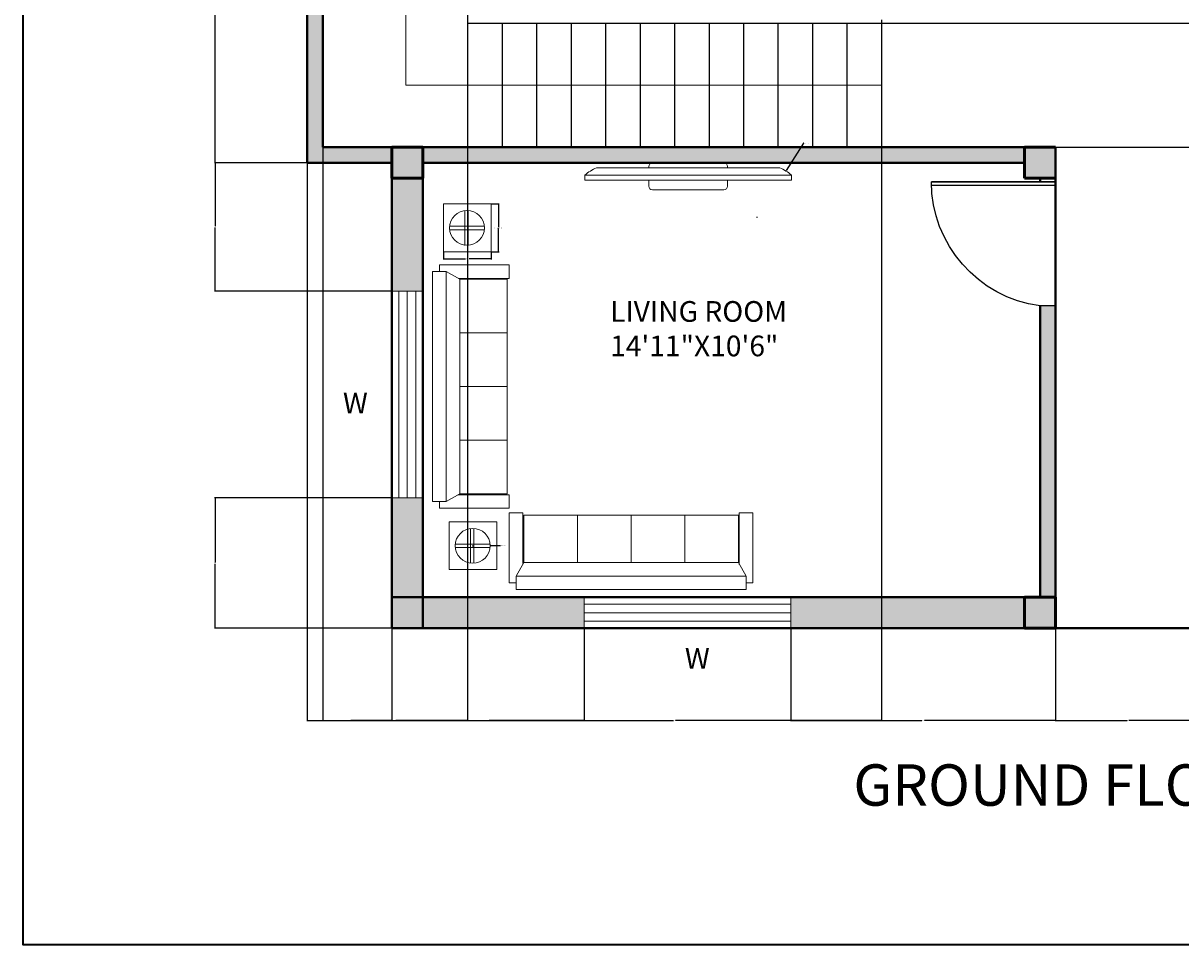
# Model space of a CAD drawing. Units: inches. Extents: x 25176543 to 25177243, y 80295576 to 80296086.
# Tile 1 of 11: x 25176543 to 25176879, y 80295576 to 80295843. Entities that reach past the tile are written whole.
import ezdxf

# ---------------------------------------------------------------- set-up
doc = ezdxf.new("R2010")
doc.units = ezdxf.units.IN
doc.header["$MEASUREMENT"] = 0
for name, color, linetype, lineweight in [('A-ANNO-DIMS', 2, 'Continuous', 18), ('A-ANNO-IDEN', 7, 'Continuous', 18), ('A-ANNO-SYMB', 7, 'Continuous', 18), ('A-ANNO-TTLB', 7, 'Continuous', 35), ('A-AREA-IDEN', 7, 'Continuous', 18), ('A-COLS', 7, 'Continuous', 50), ('A-COLS-PATT', 251, 'Continuous', 13), ('A-DOOR', 3, 'Continuous', 25), ('A-EQPM', 8, 'Continuous', 18), ('A-FLOR-STRS', 7, 'Continuous', 25), ('A-GLAZ', 4, 'Continuous', 18), ('A-WALL', 7, 'Continuous', 40), ('A-WALL-PATT', 146, 'Continuous', 13), ('furniture', 31, 'Continuous', 13)]:
    doc.layers.add(name, color=color, linetype=linetype, lineweight=lineweight)
doc.styles.get("Standard").update_dxf_attribs({"font": 'arial.ttf'})
doc.dimstyles.get("Standard").update_dxf_attribs({"dimtxt": 0.18, "dimasz": 0.18, "dimexe": 0.18, "dimexo": 0.0625, "dimgap": 0.09, "dimtad": 0, "dimtih": 1, "dimtoh": 1, "dimdec": 4, "dimzin": 0, "dimdsep": 46, "dimtxsty": 'Standard', "dimcen": 0.09, "dimadec": 0, "dimazin": 0, "dimtfac": 1, "dimtdec": 4, "dimtofl": 0, "dimtmove": 0, "dimatfit": 3, "dimfxl": 1, "dimtolj": 1, "dimtzin": 0, "dimarcsym": 0})

# ---------------------------------------------------------------- blocks, each defined once
blk = doc.blocks.new('SOFA-FOUR-SEAT')
for p, q in [((1.96, 70.61), (22.23, 70.61)), ((1.96, 70.61), (1.96, 68.65)), ((22.23, 66.69), (22.23, 70.61)), ((0, 68.65), (0, 1.96)), ((3.92, 68.65), (0, 68.65)), ((3.92, 68.65), (3.92, 1.96)), ((3.92, 68.65), (7.85, 66.44)), ((7.54, 66.69), (22.23, 66.69)), ((21.58, 50.87), (7.85, 50.87)), ((21.58, 35.31), (7.85, 35.31)), ((21.58, 19.74), (7.85, 19.74)), ((7.85, 4.17), (3.92, 1.96)), ((7.29, 3.92), (22.23, 3.92)), ((22.23, 3.92), (22.23, 0)), ((3.92, 1.96), (0, 1.96)), ((1.96, 1.96), (1.96, 0)), ((1.96, 0), (22.23, 0))]:
    blk.add_line(p, q)
blk.add_lwpolyline([(7.85, 66.44), (7.85, 4.17), (21.58, 4.17), (21.58, 66.44)], close=True)
blk = doc.blocks.new('END-TABLE')
for p, q in [((13.85, 13.86), (0, 13.86)), ((0, 13.86), (0, 0)), ((13.85, 0), (13.85, 13.86)), ((6.16, 11.93), (6.16, 1.84)), ((7.16, 11.93), (7.16, 1.84)), ((1.79, 7.4), (11.88, 7.4)), ((1.79, 6.4), (11.88, 6.4)), ((0, 0), (13.85, 0))]:
    blk.add_line(p, q)
blk.add_circle((6.83, 6.93), 5.05)
blk = doc.blocks.new('WIN-60IN')
for p, q in [((0, 9), (0, 0)), ((60, 9), (0, 9)), ((0, 9), (0, 4.5)), ((60, 7), (0, 7)), ((60, 0), (60, 9)), ((0, 4.5), (60, 4.5)), ((0, 2), (60, 2)), ((0, 0), (60, 0))]:
    blk.add_line(p, q)
blk = doc.blocks.new('DOOR-36IN')
for p, q in [((36, 37), (31.5, 37)), ((36, 1), (36, 37)), ((0, 2), (36, 2)), ((36, 1), (0, 1)), ((0, 1), (36, 1)), ((36, 0), (36, 1))]:
    blk.add_line(p, q)
blk.add_arc((36.32, 1), 36.32, 97.6281, 180)
blk = doc.blocks.new('COLUMN-9IN-SQ')
for p, q in [((9, 9), (0, 9)), ((0, 9), (0, 0)), ((9, 0), (9, 9)), ((0, 0), (9, 0))]:
    blk.add_line(p, q)
blk = doc.blocks.new('*D36')
at = {"layer": 'A-ANNO-DIMS', "color": 0, "lineweight": -2, "transparency": 16777216}
for p, q in [((25176678.7, 80295790.86), (25176680.9, 80295790.86)), ((25176680.72, 80295790.68), (25176680.72, 80295784.11)), ((25176680.72, 80295777.17), (25176680.72, 80295783.74)), ((25176678.7, 80295776.99), (25176680.9, 80295776.99))]:
    blk.add_line(p, q, dxfattribs=at)
at = {"layer": 'A-ANNO-DIMS', "color": 0, "transparency": 16777216}
for points in [[(25176680.69, 80295790.68), (25176680.75, 80295790.68), (25176680.72, 80295790.86)], [(25176680.69, 80295777.17), (25176680.75, 80295777.17), (25176680.72, 80295776.99)]]:
    blk.add_solid(points, dxfattribs=at)
at = {"layer": 'Defpoints', "color": 0, "transparency": 16777216}
for p in [(25176678.64, 80295790.86), (25176680.72, 80295790.86), (25176678.64, 80295776.99)]:
    blk.add_point(p, dxfattribs=at)
at = {"layer": 'A-ANNO-DIMS', "color": 0, "transparency": 16777216, "insert": (25176680.72, 80295783.92), "char_height": 0.18, "attachment_point": 5}
blk.add_mtext('\\A1;END TABLE 14 TYP.', dxfattribs=at)
blk = doc.blocks.new('*D37')
at = {"layer": 'A-ANNO-DIMS', "color": 0, "lineweight": -2, "transparency": 16777216}
for p, q in [((25176664.79, 80295776.93), (25176664.79, 80295774.74)), ((25176664.97, 80295774.92), (25176671.19, 80295774.92)), ((25176678.46, 80295774.92), (25176672.23, 80295774.92)), ((25176678.64, 80295776.93), (25176678.64, 80295774.74))]:
    blk.add_line(p, q, dxfattribs=at)
at = {"layer": 'A-ANNO-DIMS', "color": 0, "transparency": 16777216}
for points in [[(25176664.97, 80295774.95), (25176664.97, 80295774.89), (25176664.79, 80295774.92)], [(25176678.46, 80295774.95), (25176678.46, 80295774.89), (25176678.64, 80295774.92)]]:
    blk.add_solid(points, dxfattribs=at)
at = {"layer": 'Defpoints', "color": 0, "transparency": 16777216}
for p in [(25176664.79, 80295776.99), (25176678.64, 80295776.99), (25176678.64, 80295774.92)]:
    blk.add_point(p, dxfattribs=at)
at = {"layer": 'A-ANNO-DIMS', "color": 0, "transparency": 16777216, "insert": (25176671.71, 80295774.92), "char_height": 0.18, "attachment_point": 5}
blk.add_mtext('\\A1;14 TYP.', dxfattribs=at)
blk = doc.blocks.new('*D50')
at = {"layer": 'A-ANNO-DIMS', "color": 0, "lineweight": -2, "transparency": 16777216}
for p, q in [((25176625.3, 80295802.74), (25176625.3, 80295640.87)), ((25176649.8, 80295802.74), (25176649.8, 80295640.87)), ((25176625.48, 80295641.05), (25176637.23, 80295641.05)), ((25176649.62, 80295641.05), (25176637.88, 80295641.05))]:
    blk.add_line(p, q, dxfattribs=at)
at = {"layer": 'A-ANNO-DIMS', "color": 0, "transparency": 16777216}
for points in [[(25176625.48, 80295641.08), (25176625.48, 80295641.02), (25176625.3, 80295641.05)], [(25176649.62, 80295641.08), (25176649.62, 80295641.02), (25176649.8, 80295641.05)]]:
    blk.add_solid(points, dxfattribs=at)
at = {"layer": 'Defpoints', "color": 0, "transparency": 16777216}
for p in [(25176625.3, 80295802.8), (25176649.8, 80295802.8), (25176649.8, 80295641.05)]:
    blk.add_point(p, dxfattribs=at)
at = {"layer": 'A-ANNO-DIMS', "color": 0, "transparency": 16777216, "insert": (25176637.55, 80295641.05), "char_height": 0.18, "attachment_point": 5}
blk.add_mtext('\\A1;24.5', dxfattribs=at)
blk = doc.blocks.new('*D51')
at = {"layer": 'A-ANNO-DIMS', "color": 0, "lineweight": -2, "transparency": 16777216}
for p, q in [((25176625.24, 80295890.3), (25176598.37, 80295890.3)), ((25176598.55, 80295890.12), (25176598.55, 80295846.73)), ((25176598.55, 80295802.98), (25176598.55, 80295846.37)), ((25176625.24, 80295802.8), (25176598.37, 80295802.8))]:
    blk.add_line(p, q, dxfattribs=at)
at = {"layer": 'A-ANNO-DIMS', "color": 0, "transparency": 16777216}
for points in [[(25176598.52, 80295890.12), (25176598.58, 80295890.12), (25176598.55, 80295890.3)], [(25176598.52, 80295802.98), (25176598.58, 80295802.98), (25176598.55, 80295802.8)]]:
    blk.add_solid(points, dxfattribs=at)
at = {"layer": 'Defpoints', "color": 0, "transparency": 16777216}
for p in [(25176598.55, 80295890.3), (25176625.3, 80295890.3), (25176625.3, 80295802.8)]:
    blk.add_point(p, dxfattribs=at)
at = {"layer": 'A-ANNO-DIMS', "color": 0, "transparency": 16777216, "insert": (25176598.55, 80295846.55), "char_height": 0.18, "attachment_point": 5}
blk.add_mtext('\\A1;87.5', dxfattribs=at)
blk = doc.blocks.new('*D52')
at = {"layer": 'A-ANNO-DIMS', "color": 0, "lineweight": -2, "transparency": 16777216}
for p, q in [((25176842.3, 80295667.74), (25176842.3, 80295640.87)), ((25176884.3, 80295667.74), (25176884.3, 80295640.87)), ((25176842.48, 80295641.05), (25176863.08, 80295641.05)), ((25176884.12, 80295641.05), (25176863.52, 80295641.05))]:
    blk.add_line(p, q, dxfattribs=at)
at = {"layer": 'A-ANNO-DIMS', "color": 0, "transparency": 16777216}
for points in [[(25176842.48, 80295641.08), (25176842.48, 80295641.02), (25176842.3, 80295641.05)], [(25176884.12, 80295641.08), (25176884.12, 80295641.02), (25176884.3, 80295641.05)]]:
    blk.add_solid(points, dxfattribs=at)
at = {"layer": 'Defpoints', "color": 0, "transparency": 16777216}
for p in [(25176842.3, 80295667.8), (25176884.3, 80295667.8), (25176884.3, 80295641.05)]:
    blk.add_point(p, dxfattribs=at)
at = {"layer": 'A-ANNO-DIMS', "color": 0, "transparency": 16777216, "insert": (25176863.3, 80295641.05), "char_height": 0.18, "attachment_point": 5}
blk.add_mtext('\\A1;42', dxfattribs=at)
blk = doc.blocks.new('*D53')
at = {"layer": 'A-ANNO-DIMS', "color": 0, "lineweight": -2, "transparency": 16777216}
for p, q in [((25176649.8, 80295667.74), (25176649.8, 80295640.87)), ((25176705.57, 80295667.74), (25176705.57, 80295640.87)), ((25176649.98, 80295641.05), (25176677.29, 80295641.05)), ((25176705.39, 80295641.05), (25176678.08, 80295641.05))]:
    blk.add_line(p, q, dxfattribs=at)
at = {"layer": 'A-ANNO-DIMS', "color": 0, "transparency": 16777216}
for points in [[(25176649.98, 80295641.08), (25176649.98, 80295641.02), (25176649.8, 80295641.05)], [(25176705.39, 80295641.08), (25176705.39, 80295641.02), (25176705.57, 80295641.05)]]:
    blk.add_solid(points, dxfattribs=at)
at = {"layer": 'Defpoints', "color": 0, "transparency": 16777216}
for p in [(25176649.8, 80295667.8), (25176705.57, 80295667.8), (25176705.57, 80295641.05)]:
    blk.add_point(p, dxfattribs=at)
at = {"layer": 'A-ANNO-DIMS', "color": 0, "transparency": 16777216, "insert": (25176677.69, 80295641.05), "char_height": 0.18, "attachment_point": 5}
blk.add_mtext('\\A1;55.77', dxfattribs=at)
blk = doc.blocks.new('*D54')
at = {"layer": 'A-ANNO-DIMS', "color": 0, "lineweight": -2, "transparency": 16777216}
for p, q in [((25176765.57, 80295667.74), (25176765.57, 80295640.87)), ((25176842.3, 80295667.74), (25176842.3, 80295640.87)), ((25176765.75, 80295641.05), (25176803.54, 80295641.05)), ((25176842.12, 80295641.05), (25176804.33, 80295641.05))]:
    blk.add_line(p, q, dxfattribs=at)
at = {"layer": 'A-ANNO-DIMS', "color": 0, "transparency": 16777216}
for points in [[(25176765.75, 80295641.08), (25176765.75, 80295641.02), (25176765.57, 80295641.05)], [(25176842.12, 80295641.08), (25176842.12, 80295641.02), (25176842.3, 80295641.05)]]:
    blk.add_solid(points, dxfattribs=at)
at = {"layer": 'Defpoints', "color": 0, "transparency": 16777216}
for p in [(25176765.57, 80295667.8), (25176842.3, 80295667.8), (25176842.3, 80295641.05)]:
    blk.add_point(p, dxfattribs=at)
at = {"layer": 'A-ANNO-DIMS', "color": 0, "transparency": 16777216, "insert": (25176803.94, 80295641.05), "char_height": 0.18, "attachment_point": 5}
blk.add_mtext('\\A1;76.73', dxfattribs=at)
blk = doc.blocks.new('*D59')
at = {"layer": 'A-ANNO-DIMS', "color": 0, "lineweight": -2, "transparency": 16777216}
for p, q in [((25176649.74, 80295802.8), (25176598.37, 80295802.8)), ((25176598.55, 80295802.62), (25176598.55, 80295784.37)), ((25176598.55, 80295765.75), (25176598.55, 80295784)), ((25176649.74, 80295765.57), (25176598.37, 80295765.57))]:
    blk.add_line(p, q, dxfattribs=at)
at = {"layer": 'A-ANNO-DIMS', "color": 0, "transparency": 16777216}
for points in [[(25176598.52, 80295802.62), (25176598.58, 80295802.62), (25176598.55, 80295802.8)], [(25176598.52, 80295765.75), (25176598.58, 80295765.75), (25176598.55, 80295765.57)]]:
    blk.add_solid(points, dxfattribs=at)
at = {"layer": 'Defpoints', "color": 0, "transparency": 16777216}
for p in [(25176598.55, 80295802.8), (25176649.8, 80295802.8), (25176649.8, 80295765.57)]:
    blk.add_point(p, dxfattribs=at)
at = {"layer": 'A-ANNO-DIMS', "color": 0, "transparency": 16777216, "insert": (25176598.55, 80295784.19), "char_height": 0.18, "attachment_point": 5}
blk.add_mtext('\\A1;37.23', dxfattribs=at)
blk = doc.blocks.new('*D60')
at = {"layer": 'A-ANNO-DIMS', "color": 0, "lineweight": -2, "transparency": 16777216}
for p, q in [((25176649.74, 80295705.57), (25176598.37, 80295705.57)), ((25176598.55, 80295705.39), (25176598.55, 80295686.87)), ((25176598.55, 80295667.98), (25176598.55, 80295686.5)), ((25176649.74, 80295667.8), (25176598.37, 80295667.8))]:
    blk.add_line(p, q, dxfattribs=at)
at = {"layer": 'A-ANNO-DIMS', "color": 0, "transparency": 16777216}
for points in [[(25176598.52, 80295705.39), (25176598.58, 80295705.39), (25176598.55, 80295705.57)], [(25176598.52, 80295667.98), (25176598.58, 80295667.98), (25176598.55, 80295667.8)]]:
    blk.add_solid(points, dxfattribs=at)
at = {"layer": 'Defpoints', "color": 0, "transparency": 16777216}
for p in [(25176598.55, 80295705.57), (25176649.8, 80295705.57), (25176649.8, 80295667.8)]:
    blk.add_point(p, dxfattribs=at)
at = {"layer": 'A-ANNO-DIMS', "color": 0, "transparency": 16777216, "insert": (25176598.55, 80295686.69), "char_height": 0.18, "attachment_point": 5}
blk.add_mtext('\\A1;37.77', dxfattribs=at)
blk = doc.blocks.new('*D71')
at = {"layer": 'A-ANNO-DIMS', "color": 0, "lineweight": -2, "transparency": 16777216}
for p, q in [((25176671.8, 80295807.24), (25176671.8, 80295640.87)), ((25176791.8, 80295807.24), (25176791.8, 80295640.87)), ((25176671.98, 80295641.05), (25176731.52, 80295641.05)), ((25176791.62, 80295641.05), (25176732.08, 80295641.05))]:
    blk.add_line(p, q, dxfattribs=at)
at = {"layer": 'A-ANNO-DIMS', "color": 0, "transparency": 16777216}
for points in [[(25176671.98, 80295641.08), (25176671.98, 80295641.02), (25176671.8, 80295641.05)], [(25176791.62, 80295641.08), (25176791.62, 80295641.02), (25176791.8, 80295641.05)]]:
    blk.add_solid(points, dxfattribs=at)
at = {"layer": 'Defpoints', "color": 0, "transparency": 16777216}
for p in [(25176671.8, 80295807.3), (25176791.8, 80295807.3), (25176791.8, 80295641.05)]:
    blk.add_point(p, dxfattribs=at)
at = {"layer": 'A-ANNO-DIMS', "color": 0, "transparency": 16777216, "insert": (25176731.8, 80295641.05), "char_height": 0.18, "attachment_point": 5}
blk.add_mtext('\\A1;120', dxfattribs=at)
blk = doc.blocks.new('*D72')
at = {"layer": 'A-ANNO-DIMS', "color": 0, "lineweight": -2, "transparency": 16777216}
for p, q in [((25176629.8, 80295807.24), (25176629.8, 80295640.87)), ((25176671.8, 80295807.24), (25176671.8, 80295640.87)), ((25176629.98, 80295641.05), (25176650.58, 80295641.05)), ((25176671.62, 80295641.05), (25176651.02, 80295641.05))]:
    blk.add_line(p, q, dxfattribs=at)
at = {"layer": 'A-ANNO-DIMS', "color": 0, "transparency": 16777216}
for points in [[(25176629.98, 80295641.08), (25176629.98, 80295641.02), (25176629.8, 80295641.05)], [(25176671.62, 80295641.08), (25176671.62, 80295641.02), (25176671.8, 80295641.05)]]:
    blk.add_solid(points, dxfattribs=at)
at = {"layer": 'Defpoints', "color": 0, "transparency": 16777216}
for p in [(25176629.8, 80295807.3), (25176671.8, 80295807.3), (25176671.8, 80295641.05)]:
    blk.add_point(p, dxfattribs=at)
at = {"layer": 'A-ANNO-DIMS', "color": 0, "transparency": 16777216, "insert": (25176650.8, 80295641.05), "char_height": 0.18, "attachment_point": 5}
blk.add_mtext('\\A1;42', dxfattribs=at)
blk = doc.blocks.new('*D73')
at = {"layer": 'A-ANNO-DIMS', "color": 0, "lineweight": -2, "transparency": 16777216}
for p, q in [((25176791.86, 80295843.3), (25177152.73, 80295843.3)), ((25177152.55, 80295843.12), (25177152.55, 80295825.48)), ((25177152.55, 80295807.48), (25177152.55, 80295825.12)), ((25176791.86, 80295807.3), (25177152.73, 80295807.3))]:
    blk.add_line(p, q, dxfattribs=at)
at = {"layer": 'A-ANNO-DIMS', "color": 0, "transparency": 16777216}
for points in [[(25177152.52, 80295843.12), (25177152.58, 80295843.12), (25177152.55, 80295843.3)], [(25177152.52, 80295807.48), (25177152.58, 80295807.48), (25177152.55, 80295807.3)]]:
    blk.add_solid(points, dxfattribs=at)
at = {"layer": 'Defpoints', "color": 0, "transparency": 16777216}
for p in [(25176791.8, 80295843.3), (25177152.55, 80295843.3), (25176791.8, 80295807.3)]:
    blk.add_point(p, dxfattribs=at)
at = {"layer": 'A-ANNO-DIMS', "color": 0, "transparency": 16777216, "insert": (25177152.55, 80295825.3), "char_height": 0.18, "attachment_point": 5}
blk.add_mtext('\\A1;36', dxfattribs=at)
blk = doc.blocks.new('*D80')
at = {"layer": 'A-ANNO-DIMS', "color": 0, "lineweight": -2, "transparency": 16777216}
for p, q in [((25176769.16, 80295808.45), (25176764.21, 80295800.56)), ((25176769.34, 80295808.45), (25176769.16, 80295808.45)), ((25176755.63, 80295787.01), (25176755.81, 80295787.01)), ((25176755.72, 80295786.92), (25176755.72, 80295787.1))]:
    blk.add_line(p, q, dxfattribs=at)
at = {"layer": 'A-ANNO-DIMS', "color": 0, "transparency": 16777216}
blk.add_solid([(25176764.19, 80295800.58), (25176764.24, 80295800.55), (25176764.12, 80295800.41)], dxfattribs=at)
at = {"layer": 'Defpoints', "color": 0, "transparency": 16777216}
for p in [(25176764.12, 80295800.41), (25176755.72, 80295787.01)]:
    blk.add_point(p, dxfattribs=at)
at = {"layer": 'A-ANNO-DIMS', "color": 0, "transparency": 16777216, "insert": (25176770.08, 80295808.45), "char_height": 0.18, "attachment_point": 5}
blk.add_mtext('\\A1;2X R15.813', dxfattribs=at)
blk = doc.blocks.new('*D81')
at = {"layer": 'A-ANNO-DIMS', "color": 0, "lineweight": -2, "transparency": 16777216}
for p, q in [((25176673.18, 80295691.72), (25176673.36, 80295691.72)), ((25176673.27, 80295691.63), (25176673.27, 80295691.81)), ((25176681.35, 80295691.71), (25176678.5, 80295691.71))]:
    blk.add_line(p, q, dxfattribs=at)
at = {"layer": 'A-ANNO-DIMS', "color": 0, "transparency": 16777216}
blk.add_solid([(25176678.5, 80295691.74), (25176678.5, 80295691.68), (25176678.32, 80295691.71)], dxfattribs=at)
at = {"layer": 'Defpoints', "color": 0, "transparency": 16777216}
for p in [(25176668.23, 80295691.72), (25176678.32, 80295691.71)]:
    blk.add_point(p, dxfattribs=at)
at = {"layer": 'A-ANNO-DIMS', "color": 0, "transparency": 16777216, "insert": (25176682.1, 80295691.71), "char_height": 0.18, "attachment_point": 5}
blk.add_mtext('\\A1;2X ∅10.093', dxfattribs=at)

msp = doc.modelspace()

# ---------------------------------------------------------------- hatches: boundary and pattern name
at = {"layer": 'A-COLS-PATT'}
h = msp.add_hatch(color=256, dxfattribs=at)
h.dxf.hatch_style = 1
h.paths.add_polyline_path([(25176658.8016, 80296025.3022), (25176649.8016, 80296025.3022), (25176649.8016, 80296016.3022), (25176658.8016, 80296016.3022)])
h.paths.add_polyline_path([(25176819.3016, 80296025.3022), (25176810.3016, 80296025.3022), (25176810.3016, 80296016.3022), (25176819.3016, 80296016.3022)])
h.paths.add_polyline_path([(25176876.3016, 80296025.3022), (25176867.3016, 80296025.3022), (25176867.3016, 80296016.3022), (25176876.3016, 80296016.3022)])
h.paths.add_polyline_path([(25177013.3016, 80296025.3022), (25177004.3016, 80296025.3022), (25177004.3016, 80296016.3022), (25177013.3016, 80296016.3022)])
h.paths.add_polyline_path([(25176819.3016, 80295890.3022), (25176810.3016, 80295890.3022), (25176810.3016, 80295881.3022), (25176819.3016, 80295881.3022)])
h.paths.add_polyline_path([(25176658.8016, 80295890.3022), (25176649.8016, 80295890.3022), (25176649.8016, 80295881.3022), (25176658.8016, 80295881.3022)])
h.paths.add_polyline_path([(25177125.8016, 80296025.3022), (25177116.8016, 80296025.3022), (25177116.8016, 80296016.3022), (25177125.8016, 80296016.3022)])
h.paths.add_polyline_path([(25177125.8016, 80295848.3022), (25177116.8016, 80295848.3022), (25177116.8016, 80295839.3022), (25177125.8016, 80295839.3022)])
h.paths.add_polyline_path([(25177013.3016, 80295848.3022), (25177004.3016, 80295848.3022), (25177004.3016, 80295839.3022), (25177013.3016, 80295839.3022)])
h.paths.add_polyline_path([(25177125.8016, 80295676.8022), (25177116.8016, 80295676.8022), (25177116.8016, 80295667.8022), (25177125.8016, 80295667.8022)])
h.paths.add_polyline_path([(25177013.3016, 80295676.8022), (25177004.3016, 80295676.8022), (25177004.3016, 80295667.8022), (25177013.3016, 80295667.8022)])
h.paths.add_polyline_path([(25176842.3016, 80295676.8022), (25176833.3016, 80295676.8022), (25176833.3016, 80295667.8022), (25176842.3016, 80295667.8022)])
h.paths.add_polyline_path([(25176893.3016, 80295676.8022), (25176884.3016, 80295676.8022), (25176884.3016, 80295667.8022), (25176893.3016, 80295667.8022)])
h.paths.add_polyline_path([(25176842.3016, 80295807.3022), (25176833.3016, 80295807.3022), (25176833.3016, 80295798.3022), (25176842.3016, 80295798.3022)])
h.paths.add_polyline_path([(25176658.8016, 80295807.3022), (25176649.8016, 80295807.3022), (25176649.8016, 80295798.3022), (25176658.8016, 80295798.3022)])
h.paths.add_polyline_path([(25176658.8016, 80295676.8022), (25176649.8016, 80295676.8022), (25176649.8016, 80295667.8022), (25176658.8016, 80295667.8022)])
at = {"layer": 'A-WALL-PATT'}
h = msp.add_hatch(color=256, dxfattribs=at)
h.dxf.hatch_style = 1
h.paths.add_polyline_path([(25176695.189, 80296025.3022), (25176658.8016, 80296025.3022), (25176658.8016, 80296016.3022), (25176695.189, 80296016.3022)])
h.paths.add_polyline_path([(25176810.3016, 80296025.3022), (25176755.189, 80296025.3022), (25176755.189, 80296016.3022), (25176810.3016, 80296016.3022)])
h.paths.add_polyline_path([(25176819.3016, 80296016.3022), (25176814.8016, 80296016.3022), (25176814.8016, 80295965.3022), (25176819.3016, 80295965.3022)], flags=17)
h.paths.add_polyline_path([(25176828.0421, 80296025.3022), (25176819.3016, 80296025.3022), (25176819.3016, 80296016.3022), (25176828.0421, 80296016.3022)])
h.paths.add_polyline_path([(25176867.3016, 80296025.3022), (25176852.0421, 80296025.3022), (25176852.0421, 80296016.3022), (25176867.3016, 80296016.3022)])
h.paths.add_polyline_path([(25176885.1873, 80296025.3022), (25176876.3016, 80296025.3022), (25176876.3016, 80296016.3022), (25176885.1873, 80296016.3022)])
h.paths.add_polyline_path([(25176919.8016, 80296025.3022), (25176909.1873, 80296025.3022), (25176909.1873, 80296016.3022), (25176919.8016, 80296016.3022)])
h.paths.add_polyline_path([(25176924.3016, 80296016.3022), (25176919.8016, 80296016.3022), (25176919.8016, 80295890.3022), (25176904.8016, 80295890.3022), (25176904.8016, 80295885.8022), (25176967.3016, 80295885.8022), (25176967.3016, 80295890.3022), (25176924.3016, 80295890.3022)])
h.paths.add_polyline_path([(25176924.3016, 80296025.3022), (25176919.8016, 80296025.3022), (25176919.8016, 80296016.3022), (25176924.3016, 80296016.3022)])
h.paths.add_polyline_path([(25176938.7147, 80296025.3022), (25176924.3016, 80296025.3022), (25176924.3016, 80296016.3022), (25176938.7147, 80296016.3022)])
h.paths.add_polyline_path([(25176871.8016, 80296016.3022), (25176867.3016, 80296016.3022), (25176867.3016, 80295932.3022), (25176819.3016, 80295932.3022), (25176819.3016, 80295933.3022), (25176814.8016, 80295933.3022), (25176814.8016, 80295932.3022), (25176814.8016, 80295927.3022), (25176819.3016, 80295927.3022), (25176819.3016, 80295927.8022), (25176867.3016, 80295927.8022), (25176867.3016, 80295885.8022), (25176871.8016, 80295885.8022), (25176872.8016, 80295885.8022), (25176872.8016, 80295890.3022), (25176871.8016, 80295890.3022)])
h.paths.add_polyline_path([(25177004.3016, 80296025.3022), (25176986.7147, 80296025.3022), (25176986.7147, 80296016.3022), (25177004.3016, 80296016.3022)])
h.paths.add_polyline_path([(25177035.845, 80296025.3022), (25177013.3016, 80296025.3022), (25177013.3016, 80296016.3022), (25177035.845, 80296016.3022)])
h.paths.add_polyline_path([(25177008.8016, 80296016.3022), (25177004.3016, 80296016.3022), (25177004.3016, 80295890.3022), (25177003.3016, 80295890.3022), (25177003.3016, 80295885.8022), (25177004.3016, 80295885.8022), (25177004.3016, 80295885.3022), (25177008.8016, 80295885.3022)])
h.paths.add_polyline_path([(25177116.8016, 80296025.3022), (25177095.845, 80296025.3022), (25177095.845, 80296016.3022), (25177116.8016, 80296016.3022)])
h.paths.add_polyline_path([(25177125.8016, 80296016.3022), (25177116.8016, 80296016.3022), (25177116.8016, 80295971.1334), (25177121.3016, 80295971.1334), (25177125.8016, 80295971.1334)])
h.paths.add_polyline_path([(25177116.8016, 80295848.3022), (25177013.3016, 80295848.3022), (25177013.3016, 80295843.8022), (25177116.8016, 80295843.8022)])
h.paths.add_polyline_path([(25177125.8016, 80295911.1334), (25177116.8016, 80295911.1334), (25177116.8016, 80295848.3022), (25177125.8016, 80295848.3022)])
h.paths.add_polyline_path([(25177008.8016, 80295802.3022), (25177004.3016, 80295802.3022), (25177004.3016, 80295676.8022), (25177008.8016, 80295676.8022)])
h.paths.add_polyline_path([(25176658.8016, 80295705.5694), (25176649.8016, 80295705.5694), (25176649.8016, 80295676.8022), (25176658.8016, 80295676.8022)])
h.paths.add_polyline_path([(25176658.8016, 80295798.3022), (25176649.8016, 80295798.3022), (25176649.8016, 80295765.5694), (25176654.3016, 80295765.5694), (25176658.8016, 80295765.5694)])
h.paths.add_polyline_path([(25176833.3016, 80295807.3022), (25176658.8016, 80295807.3022), (25176658.8016, 80295802.8022), (25176833.3016, 80295802.8022)])
h.paths.add_polyline_path([(25176842.3016, 80295761.3022), (25176837.8016, 80295761.3022), (25176837.8016, 80295676.8022), (25176842.3016, 80295676.8022)])
h.paths.add_polyline_path([(25176649.8016, 80295807.3022), (25176629.8016, 80295807.3022), (25176629.8016, 80295885.8022), (25176649.8016, 80295885.8022), (25176649.8016, 80295890.3022), (25176625.3016, 80295890.3022), (25176625.3016, 80295802.8022), (25176649.8016, 80295802.8022)])
h.paths.add_polyline_path([(25176810.3016, 80295890.3022), (25176658.8016, 80295890.3022), (25176658.8016, 80295885.8022), (25176810.3016, 80295885.8022)])
h.paths.add_polyline_path([(25176658.8016, 80295922.9263), (25176649.8016, 80295922.9263), (25176649.8016, 80295890.3022), (25176658.8016, 80295890.3022)])
h.paths.add_polyline_path([(25176658.8016, 80296016.3022), (25176649.8016, 80296016.3022), (25176649.8016, 80295982.9263), (25176654.3016, 80295982.9263), (25176658.8016, 80295982.9263)])
h = msp.add_hatch(color=256, dxfattribs=at)
h.dxf.hatch_style = 1
h.paths.add_polyline_path([(25176705.5738, 80295676.8022), (25176658.8016, 80295676.8022), (25176658.8016, 80295667.8022), (25176705.5738, 80295667.8022)])
h.paths.add_polyline_path([(25176833.3016, 80295676.8022), (25176765.5738, 80295676.8022), (25176765.5738, 80295667.8022), (25176833.3016, 80295667.8022)])
h.paths.add_polyline_path([(25176925.2997, 80295676.8022), (25176893.3016, 80295676.8022), (25176893.3016, 80295667.8022), (25176925.2997, 80295667.8022)])
h.paths.add_polyline_path([(25177004.3016, 80295676.8022), (25176985.2997, 80295676.8022), (25176985.2997, 80295667.8022), (25177004.3016, 80295667.8022)])
h.paths.add_polyline_path([(25177030.5901, 80295676.8022), (25177013.3016, 80295676.8022), (25177013.3016, 80295667.8022), (25177030.5901, 80295667.8022)])
h.paths.add_polyline_path([(25177116.8016, 80295676.8022), (25177090.5901, 80295676.8022), (25177090.5901, 80295667.8022), (25177116.8016, 80295667.8022)])
h.paths.add_polyline_path([(25177125.8016, 80295729.6384), (25177116.8016, 80295729.6384), (25177116.8016, 80295676.8022), (25177125.8016, 80295676.8022)])
h.paths.add_polyline_path([(25177125.8016, 80295839.3022), (25177116.8016, 80295839.3022), (25177116.8016, 80295789.6384), (25177121.3016, 80295789.6384), (25177125.8016, 80295789.6384)])

# ---------------------------------------------------------------- linework, layer by layer
at = {"layer": 'A-ANNO-SYMB'}
for p, q in [((25176653.8935, 80295825.3022), (25176653.8935, 80295865.9686)), ((25176791.8016, 80295825.3022), (25176653.8935, 80295825.3022))]:
    msp.add_line(p, q, dxfattribs=at)
at = {"layer": 'A-ANNO-TTLB'}
msp.add_lwpolyline([(25176542.8973, 80296086.2335), (25177242.9194, 80296086.2335), (25177242.9194, 80295575.9501), (25176542.8973, 80295575.9501)], close=True, dxfattribs=at)
at = {"layer": 'A-COLS'}
for p, q in [((25176842.3016, 80295807.3022), (25176833.3016, 80295807.3022)), ((25176833.3016, 80295807.3022), (25176833.3016, 80295798.3022)), ((25176833.3016, 80295798.3022), (25176842.3016, 80295798.3022))]:
    msp.add_line(p, q, dxfattribs=at)
at = {"layer": 'A-EQPM'}
for p, q in [((25176709.1673, 80295801.3735), (25176762.3389, 80295801.3735)), ((25176724.3231, 80295801.3735), (25176724.3231, 80295801.7388)), ((25176725.3865, 80295802.8022), (25176746.1197, 80295802.8022)), ((25176747.1831, 80295801.3735), (25176747.1831, 80295801.7388)), ((25176705.7494, 80295799.2303), (25176765.7569, 80295799.2303)), ((25176705.7494, 80295799.2303), (25176705.7494, 80295797.8016)), ((25176705.7494, 80295797.8016), (25176765.7569, 80295797.8016)), ((25176724.3231, 80295797.8016), (25176724.3231, 80295796.0075)), ((25176747.1831, 80295797.8016), (25176747.1831, 80295796.0075)), ((25176765.7569, 80295799.2303), (25176765.7569, 80295797.8016)), ((25176725.3865, 80295794.9441), (25176746.1197, 80295794.9441))]:
    msp.add_line(p, q, dxfattribs=at)
for centre, radius, start, end in [((25176715.7901, 80295787.0141), 15.813, 114.760192, 129.417488), ((25176725.3865, 80295801.7388), 1.0634, 90, 180), ((25176746.1197, 80295801.7388), 1.0634, 0, 90), ((25176755.7161, 80295787.0141), 15.813, 50.582512, 65.239808), ((25176725.3865, 80295796.0075), 1.0634, 180, 270), ((25176746.1197, 80295796.0075), 1.0634, 270, 0)]:
    msp.add_arc(centre, radius, start, end, dxfattribs=at)
at = {"layer": 'A-FLOR-STRS'}
for p, q in [((25176671.8016, 80295849.8022), (25176671.8016, 80295807.3022)), ((25176671.8016, 80295843.3022), (25176791.8016, 80295843.3022)), ((25176681.8016, 80295843.3022), (25176681.8016, 80295807.3022)), ((25176691.8016, 80295843.3022), (25176691.8016, 80295807.3022)), ((25176701.8016, 80295843.3022), (25176701.8016, 80295807.3022)), ((25176711.8016, 80295843.3022), (25176711.8016, 80295807.3022)), ((25176721.8016, 80295843.3022), (25176721.8016, 80295807.3022)), ((25176731.8016, 80295843.3022), (25176731.8016, 80295807.3022)), ((25176741.8016, 80295843.3022), (25176741.8016, 80295807.3022)), ((25176751.8016, 80295843.3022), (25176751.8016, 80295807.3022)), ((25176761.8016, 80295843.3022), (25176761.8016, 80295807.3022)), ((25176771.8016, 80295843.3022), (25176771.8016, 80295807.3022)), ((25176781.8016, 80295843.3022), (25176781.8016, 80295807.3022)), ((25176791.8016, 80295844.3022), (25176791.8016, 80295843.3022)), ((25176791.8016, 80295843.3022), (25176791.8016, 80295807.3022))]:
    msp.add_line(p, q, dxfattribs=at)
at = {"layer": 'A-WALL'}
for p, q in [((25176625.3016, 80295890.3022), (25176625.3016, 80295802.8022)), ((25176629.8016, 80295885.8022), (25176629.8016, 80295807.3022)), ((25176629.8016, 80295807.3022), (25176649.8016, 80295807.3022)), ((25176649.8016, 80295807.3022), (25176842.3016, 80295807.3022)), ((25176649.8016, 80295807.3022), (25176649.8016, 80295667.8022)), ((25176658.8016, 80295807.3022), (25176658.8016, 80295667.8022)), ((25176842.3016, 80295807.3022), (25176842.3016, 80295667.8022)), ((25176842.3016, 80295807.3022), (25176842.3016, 80295807.3022)), ((25176625.3016, 80295802.8022), (25176649.8016, 80295802.8022)), ((25176658.8016, 80295802.8022), (25176833.3016, 80295802.8022)), ((25176837.8016, 80295798.3022), (25176837.8016, 80295797.3022)), ((25176842.3016, 80295798.3022), (25176842.3016, 80295797.6427)), ((25176837.8016, 80295761.3022), (25176837.8016, 80295676.8022)), ((25176649.8016, 80295676.8022), (25176842.3016, 80295676.8022)), ((25176842.3016, 80295676.8022), (25176842.3016, 80295676.8022)), ((25176649.8016, 80295667.8022), (25177125.8016, 80295667.8022)), ((25176842.3016, 80295667.8022), (25176878.3016, 80295667.8022)), ((25176878.3016, 80295667.8022), (25176884.3016, 80295667.8022))]:
    msp.add_line(p, q, dxfattribs=at)

# ---------------------------------------------------------------- block references
at = {"layer": 'A-COLS'}
for p, rotation in [((25176658.8018, 80295798.3026), 90.00000002371594), ((25176842.3018, 80295667.8026), 90.00000004743185)]:
    msp.add_blockref('COLUMN-9IN-SQ', p, dxfattribs=dict(at, rotation=rotation))
at = {"layer": 'A-DOOR', "extrusion": (0, 0, -1), "zscale": -1, "rotation": 180}
msp.add_blockref('DOOR-36IN', (-25176806.302, 80295798.3024), dxfattribs=at)
at = {"layer": 'A-GLAZ', "extrusion": (0, 0, -1), "zscale": -1, "rotation": 270.0000000443287}
msp.add_blockref('WIN-60IN', (-25176658.8018, 80295765.5695), dxfattribs=at)
at = {"layer": 'A-GLAZ'}
msp.add_blockref('WIN-60IN', (25176705.5737, 80295667.802), dxfattribs=at)
at = {"layer": 'furniture'}
for name, p in [('END-TABLE', (25176664.785, 80295776.995)), ('SOFA-FOUR-SEAT', (25176661.652, 80295702.58)), ('END-TABLE', (25176666.4424, 80295684.7855))]:
    msp.add_blockref(name, p, dxfattribs=at)
at = {"layer": 'furniture', "rotation": 90.00000004435555}
msp.add_blockref('SOFA-FOUR-SEAT', (25176754.4915, 80295679.0027), dxfattribs=at)

# ---------------------------------------------------------------- texts
at = {"layer": 'A-ANNO-IDEN', "char_height": 6, "attachment_point": 1}
for insert in [(25176635.6482, 80295736.0995), (25176734.8175, 80295662.0191)]:
    msp.add_mtext_dynamic_manual_height_columns('W', width=24.139595, gutter_width=1, heights=[0], dxfattribs=dict(at, insert=insert))
at = {"layer": 'A-ANNO-TTLB', "insert": (25176783.6607, 80295628.3104), "char_height": 12, "attachment_point": 1}
msp.add_mtext_dynamic_manual_height_columns('GROUND FLOOR PLAN', width=295.824021, gutter_width=1, heights=[0], dxfattribs=at)
at = {"layer": 'A-AREA-IDEN', "insert": (25176713.1163, 80295762.6767), "char_height": 6, "attachment_point": 1}
msp.add_mtext_dynamic_manual_height_columns('LIVING ROOM\\P14\'11"X10\'6"', width=61.585319, gutter_width=1, heights=[0], dxfattribs=at)

# ---------------------------------------------------------------- dimensions: what is measured, and where the dimension line sits
at = {"layer": 'A-ANNO-DIMS'}
for base, p1, p2, override, picture, middle in [((25176598.5516, 80295890.3022), (25176625.3016, 80295802.8022), (25176625.3016, 80295890.3022), {"dimdec": 1, "dimlfac": 1, "dimrnd": 0, "dimzin": 0, "dimdsep": 46, "dimlunit": 2}, '*D51', (25176598.5516, 80295846.5522)), ((25177152.5516, 80295843.3022), (25176791.8016, 80295807.3022), (25176791.8016, 80295843.3022), {"dimdec": 0, "dimlfac": 1, "dimrnd": 0, "dimzin": 0, "dimdsep": 46, "dimlunit": 2}, '*D73', (25177152.5516, 80295825.3022)), ((25176598.5516, 80295802.8022), (25176649.8016, 80295765.5694), (25176649.8016, 80295802.8022), {"dimdec": 2, "dimlfac": 1, "dimrnd": 0, "dimzin": 0, "dimdsep": 46, "dimlunit": 2}, '*D59', (25176598.5516, 80295784.1858)), ((25176598.5516, 80295705.5694), (25176649.8016, 80295667.8022), (25176649.8016, 80295705.5694), {"dimdec": 2, "dimlfac": 1, "dimrnd": 0, "dimzin": 0, "dimdsep": 46, "dimlunit": 2}, '*D60', (25176598.5516, 80295686.6858))]:
    dim = msp.add_linear_dim(base=base, p1=p1, p2=p2, angle=90, dimstyle='Standard', override=override, dxfattribs=at)
    dim.commit()
    dim.dimension.update_dxf_attribs({"geometry": picture, "text_midpoint": middle})
dim = msp.add_radius_dim(center=(25176755.7161, 80295787.0141), mpoint=(25176764.117, 80295800.411), text='2X <>', dimstyle='Standard', override={"dimdec": 3, "dimlfac": 1, "dimrnd": 0, "dimzin": 0, "dimdsep": 46, "dimlunit": 2}, dxfattribs=at)
dim.commit()
dim.dimension.update_dxf_attribs({"geometry": '*D80', "text_midpoint": (25176770.0823, 80295808.4492), "dimtype": 164})
for base, p1, p2, override, picture, middle in [((25176671.8016, 80295641.0522), (25176629.8016, 80295807.3022), (25176671.8016, 80295807.3022), {"dimdec": 0, "dimlfac": 1, "dimrnd": 0, "dimzin": 0, "dimdsep": 46, "dimlunit": 2}, '*D72', (25176650.8016, 80295641.0522)), ((25176791.8016, 80295641.0522), (25176671.8016, 80295807.3022), (25176791.8016, 80295807.3022), {"dimdec": 0, "dimlfac": 1, "dimrnd": 0, "dimzin": 0, "dimdsep": 46, "dimlunit": 2}, '*D71', (25176731.8016, 80295641.0522)), ((25176649.8016, 80295641.0522), (25176625.3016, 80295802.8022), (25176649.8016, 80295802.8022), {"dimdec": 1, "dimlfac": 1, "dimrnd": 0, "dimzin": 0, "dimdsep": 46, "dimlunit": 2}, '*D50', (25176637.5516, 80295641.0522)), ((25176705.5738, 80295641.0522), (25176649.8016, 80295667.8022), (25176705.5738, 80295667.8022), {"dimdec": 2, "dimlfac": 1, "dimrnd": 0, "dimzin": 0, "dimdsep": 46, "dimlunit": 2}, '*D53', (25176677.6877, 80295641.0522)), ((25176842.3016, 80295641.0522), (25176765.5738, 80295667.8022), (25176842.3016, 80295667.8022), {"dimdec": 2, "dimlfac": 1, "dimrnd": 0, "dimzin": 0, "dimdsep": 46, "dimlunit": 2}, '*D54', (25176803.9377, 80295641.0522)), ((25176884.3016, 80295641.0522), (25176842.3016, 80295667.8022), (25176884.3016, 80295667.8022), {"dimdec": 0, "dimlfac": 1, "dimrnd": 0, "dimzin": 0, "dimdsep": 46, "dimlunit": 2}, '*D52', (25176863.3016, 80295641.0522))]:
    dim = msp.add_linear_dim(base=base, p1=p1, p2=p2, dimstyle='Standard', override=override, dxfattribs=at)
    dim.commit()
    dim.dimension.update_dxf_attribs({"geometry": picture, "text_midpoint": middle})
dim = msp.add_linear_dim(base=(25176680.7179, 80295790.8551), p1=(25176678.6389, 80295776.9947), p2=(25176678.6389, 80295790.8551), angle=90, text='END TABLE <> TYP.', dimstyle='Standard', override={"dimdec": 0, "dimlfac": 1, "dimrnd": 0, "dimzin": 0, "dimdsep": 46, "dimlunit": 2}, dxfattribs=at)
dim.commit()
dim.dimension.update_dxf_attribs({"geometry": '*D36', "text_midpoint": (25176680.7179, 80295783.9249)})
dim = msp.add_linear_dim(base=(25176678.6389, 80295774.9157), p1=(25176664.7855, 80295776.9947), p2=(25176678.6389, 80295776.9947), text='<> TYP.', dimstyle='Standard', override={"dimdec": 0, "dimlfac": 1, "dimrnd": 0, "dimzin": 0, "dimdsep": 46, "dimlunit": 2}, dxfattribs=at)
dim.commit()
dim.dimension.update_dxf_attribs({"geometry": '*D37', "text_midpoint": (25176671.7122, 80295774.9157)})
dim = msp.add_diameter_dim_2p(p1=(25176668.2279, 80295691.716), p2=(25176678.3206, 80295691.715), text='2X <>', dimstyle='Standard', override={"dimdec": 3, "dimlfac": 1, "dimrnd": 0, "dimzin": 0, "dimdsep": 46, "dimlunit": 2}, dxfattribs=at)
dim.commit()
dim.dimension.update_dxf_attribs({"geometry": '*D81', "text_midpoint": (25176681.3484, 80295691.7147), "dimtype": 163})

doc.saveas('drawing.dxf')
